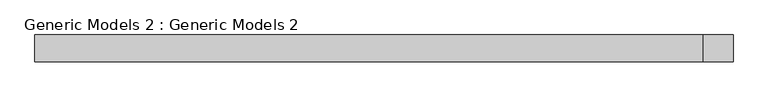
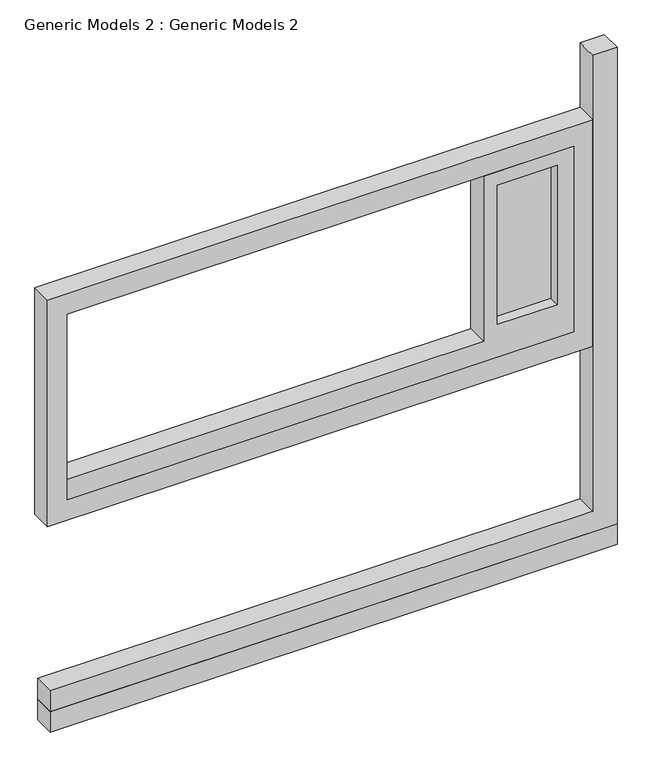
"""IFC4 building model written with IfcOpenShell, lengths in millimetres: proxy geometry, Generic Models 2 : Generic Models 2."""

from ifc_helpers import new_model, si_unit, frame, origin, place, context, project, spatial, polyline, outline, extrude, faceted_brep, source, transform, mapped, element, save


def generic_models_2_generic_models_2_cc0d390d(model_context):
    return source(origin(), model_context, "Body", "SolidModel", [
        faceted_brep([(-10112.5254541, -13854.1538163, 9144.0), (-10112.5254541, -14158.9538163, 9144.0), (-8850.5011821, -14158.9538163, 9144.0), (-8850.5011821, -13854.1538163, 9144.0), (-10112.5254541, -13854.1538163, 6705.6), (-10112.5254541, -14158.9538163, 6705.6), (-15932.2432214, -14158.9538163, 6705.6), (-15932.2432214, -14158.9538163, 6400.8), (-8850.5011821, -14158.9538163, 6400.8), (-9083.9632912, -14158.9538163, 8944.7118928), (-9083.9632912, -14158.9538163, 6887.3118928), (-9922.1632912, -14158.9538163, 6887.3118928), (-9922.1632912, -14158.9538163, 8944.7118928), (-8850.5011821, -13854.1538163, 6400.8), (-15932.2432214, -13854.1538163, 6400.8), (-15932.2432214, -13854.1538163, 6705.6), (-9083.9632912, -14006.5538163, 8944.7118928), (-9922.1632912, -14006.5538163, 8944.7118928), (-9922.1632912, -14006.5538163, 6887.3118928), (-9083.9632912, -14006.5538163, 6887.3118928)], [[[0, 1, 2, 3]], [[1, 0, 4, 5]], [[2, 1, 5, 6, 7, 8], [9, 10, 11, 12]], [[3, 2, 8, 13]], [[0, 3, 13, 14, 15, 4]], [[16, 17, 18, 19]], [[16, 19, 10, 9]], [[19, 18, 11, 10]], [[18, 17, 12, 11]], [[17, 16, 9, 12]], [[15, 6, 5, 4]], [[8, 7, 14, 13]], [[6, 15, 14, 7]]]),
        faceted_brep([(-15932.2432214, -14158.9538163, 9144.0), (-15932.2432214, -14158.9538163, 6400.8), (-15932.2432214, -13854.1538163, 6400.8), (-15932.2432214, -13854.1538163, 9144.0), (-8586.8607234, -13854.1538163, 6096.0), (-16208.891855, -13854.1538163, 6096.0), (-16208.891855, -13854.1538163, 9448.8), (-8586.8607234, -13854.1538163, 9448.8), (-8850.5011821, -13854.1538163, 6400.8), (-8850.5011821, -13854.1538163, 9144.0), (-16208.891855, -14158.9538163, 9448.8), (-16208.891855, -14158.9538163, 6096.0), (-8586.8607234, -14158.9538163, 9448.8), (-13059.291855, -14158.9538163, 9448.8), (-8586.8607234, -14158.9538163, 6096.0), (-8850.5011821, -14158.9538163, 9144.0), (-8850.5011821, -14158.9538163, 6400.8), (-8586.8607234, -14006.5538163, 9448.8)], [[[0, 1, 2, 3]], [[4, 5, 6, 7], [3, 2, 8, 9]], [[10, 6, 5, 11]], [[12, 13, 10, 11, 14], [1, 0, 15, 16]], [[12, 14, 4, 7, 17]], [[10, 13, 12, 17, 7, 6]], [[0, 3, 9, 15]], [[2, 1, 16, 8]], [[14, 11, 5, 4]], [[9, 8, 16, 15]]]),
        faceted_brep([(-16170.791855, -13854.1538163, 3657.6), (-16170.791855, -14158.9538163, 3657.6), (-8586.8607234, -14158.9538163, 3657.6), (-8586.8607234, -13854.1538163, 3657.6), (-8245.991855, -14158.9538163, 3352.8), (-16170.791855, -14158.9538163, 3352.8), (-16170.791855, -13854.1538163, 3352.8), (-8245.991855, -13854.1538163, 3352.8), (-8245.991855, -13854.1538163, 10395.767225), (-8245.991855, -14158.9538163, 10395.767225), (-8586.8607234, -13854.1538163, 10395.767225), (-8586.8607234, -14158.9538163, 10395.767225), (-8586.8607234, -14158.9538163, 9448.8), (-8586.8607234, -14006.5538163, 10395.767225)], [[[0, 1, 2, 3]], [[4, 5, 6, 7]], [[4, 7, 8, 9]], [[0, 3, 10, 8, 7, 6]], [[1, 0, 6, 5]], [[2, 1, 5, 4, 9, 11, 12]], [[9, 8, 10, 13, 11]], [[3, 2, 12, 11, 13, 10]]]),
        extrude(outline(polyline([(-8245.991855, -14158.9538163), (-16170.791855, -14158.9538163), (-16170.791855, -13854.1538163), (-8245.991855, -13854.1538163), (-8245.991855, -14158.9538163)])), frame((0.0, 0.0, 3048.0), z_axis=(0.0, 0.0, 1.0), x_axis=(1.0, 0.0, 0.0)), (0.0, 0.0, 1.0), 304.8),
    ])


if __name__ == "__main__":
    model = new_model("IFC4")
    model_context = context("Model", 3, world=origin())
    ifc_project = project(units=[si_unit("LENGTHUNIT", "METRE", prefix="MILLI")], contexts=[model_context])
    site = spatial("IfcSite", under=ifc_project)
    building = spatial("IfcBuilding", under=site)
    placement = place(None, origin())
    generic_models_2_generic_models_2_shape = generic_models_2_generic_models_2_cc0d390d(model_context)
    element("IfcBuildingElementProxy", 1, Name="Generic Models 2 : Generic Models 2", ObjectType="Generic Models 2 : Generic Models 2", at=placement, inside=building, context=model_context, shape_type="MappedRepresentation", body=[
        mapped(generic_models_2_generic_models_2_shape, transform((0.0, 0.0, 0.0), x_axis=(1.0, 0.0, 0.0), y_axis=(0.0, 1.0, 0.0), z_axis=(0.0, 0.0, 1.0))),
    ])
    save(model, "model.ifc")
